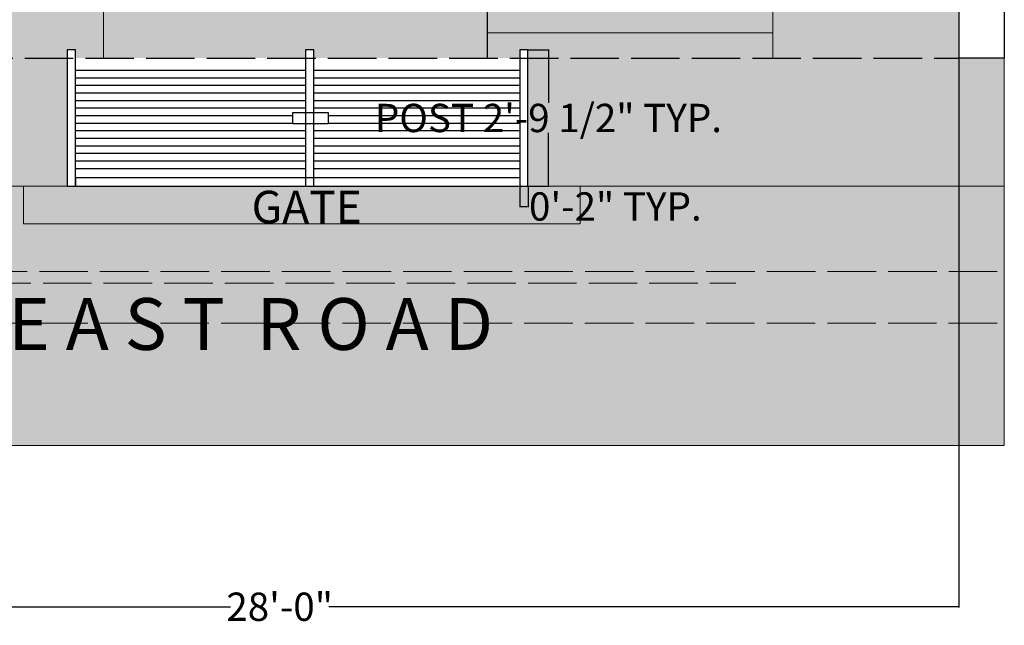
# Model space of a CAD drawing. Units: inches. Extents: x 1316 to 1777, y 813 to 1650.
# Tile 2 of 22: x 1481 to 1724, y 813 to 963. Entities that reach past the tile are written whole.
import ezdxf

# ---------------------------------------------------------------- set-up
doc = ezdxf.new("R2010")
doc.units = ezdxf.units.IN
doc.header["$MEASUREMENT"] = 0
doc.linetypes.add('ACAD_ISO02W100', pattern=[15, 12, -3])
for name, color, linetype, lineweight in [('A-ANNO-DIMS', 2, 'Continuous', 18), ('A-FLOR-STRS', 7, 'Continuous', 25), ('A-FLOR-STRS-PATT', 252, 'Continuous', 13), ('C-PROP', 8, 'ACAD_ISO02W100', 25), ('C-ROAD', 8, 'Continuous', 18), ('C-ROAD-MARK', 9, 'ACAD_ISO02W100', 13), ('C-ROAD-PATT', 251, 'Continuous', 13), ('L-HRDS', 8, 'Continuous', 18), ('L-HRDS-PATT', 252, 'Continuous', 13), ('L-SITE-GATE', 8, 'Continuous', 25), ('text', 7, 'Continuous', 18)]:
    doc.layers.add(name, color=color, linetype=linetype, lineweight=lineweight)
doc.styles.get("Standard").update_dxf_attribs({"font": 'arial.ttf'})
doc.dimstyles.get("Standard").update_dxf_attribs({"dimtxt": 7, "dimasz": 0.18, "dimexe": 0.18, "dimexo": 0.0625, "dimgap": 0.09, "dimtad": 0, "dimtih": 1, "dimtoh": 1, "dimzin": 0, "dimdsep": 46, "dimlunit": 3, "dimtxsty": 'Standard', "dimcen": 0.09, "dimadec": 0, "dimazin": 0, "dimtfac": 1, "dimtofl": 0, "dimtmove": 0, "dimatfit": 3, "dimfxl": 1, "dimtolj": 1, "dimtzin": 0, "dimarcsym": 0})

# ---------------------------------------------------------------- blocks, each defined once
blk = doc.blocks.new('GATE-END-POST')
for p, q in [((2.04, 33.69), (0, 33.69)), ((0, 33.69), (0, 31.67)), ((0, 31.67), (0, 0)), ((2.04, 31.67), (2.04, 33.69)), ((2.04, 0), (2.04, 31.67)), ((0, 0), (2.04, 0))]:
    blk.add_line(p, q)
blk = doc.blocks.new('*D38')
at = {"layer": 'A-ANNO-DIMS', "color": 0, "lineweight": -2, "transparency": 16777216}
for p, q in [((1606.62, 955.71), (1611.79, 955.71)), ((1611.61, 955.53), (1611.61, 942.57)), ((1611.61, 922.2), (1611.61, 935.15)), ((1606.62, 922.02), (1611.79, 922.02))]:
    blk.add_line(p, q, dxfattribs=at)
at = {"layer": 'A-ANNO-DIMS', "color": 0, "transparency": 16777216}
for points in [[(1611.58, 955.53), (1611.64, 955.53), (1611.61, 955.71)], [(1611.58, 922.2), (1611.64, 922.2), (1611.61, 922.02)]]:
    blk.add_solid(points, dxfattribs=at)
at = {"layer": 'Defpoints', "color": 0, "transparency": 16777216}
for p in [(1606.56, 955.71), (1611.61, 955.71), (1606.56, 922.02)]:
    blk.add_point(p, dxfattribs=at)
at = {"layer": 'A-ANNO-DIMS', "color": 0, "transparency": 16777216, "insert": (1611.61, 938.86), "char_height": 7, "attachment_point": 5}
blk.add_mtext('\\A1;POST 2\'-9 1/2" TYP.', dxfattribs=at)
blk = doc.blocks.new('*D39')
at = {"layer": 'A-ANNO-DIMS', "color": 0, "lineweight": -2, "transparency": 16777216}
for p, q in [((1604.52, 921.96), (1604.52, 916.79)), ((1606.56, 921.96), (1606.56, 916.79)), ((1604.7, 916.97), (1606.38, 916.97)), ((1606.56, 916.97), (1606.74, 916.97))]:
    blk.add_line(p, q, dxfattribs=at)
at = {"layer": 'A-ANNO-DIMS', "color": 0, "transparency": 16777216}
for points in [[(1604.7, 917), (1604.7, 916.94), (1604.52, 916.97)], [(1606.38, 917), (1606.38, 916.94), (1606.56, 916.97)]]:
    blk.add_solid(points, dxfattribs=at)
at = {"layer": 'Defpoints', "color": 0, "transparency": 16777216}
for p in [(1604.52, 922.02), (1606.56, 922.02), (1606.56, 916.97)]:
    blk.add_point(p, dxfattribs=at)
at = {"layer": 'A-ANNO-DIMS', "color": 0, "transparency": 16777216, "insert": (1628.17, 916.97), "char_height": 7, "attachment_point": 5}
blk.add_mtext('\\A1;0\'-2" TYP.', dxfattribs=at)
blk = doc.blocks.new('*D50')
at = {"layer": 'A-ANNO-DIMS', "color": 0, "lineweight": -2, "transparency": 16777216}
for p, q in [((1377.06, 1063.81), (1377.06, 817.77)), ((1713.17, 1031.11), (1713.17, 817.77)), ((1377.24, 817.95), (1532.95, 817.95)), ((1712.99, 817.95), (1557.29, 817.95))]:
    blk.add_line(p, q, dxfattribs=at)
at = {"layer": 'A-ANNO-DIMS', "color": 0, "transparency": 16777216}
for points in [[(1377.24, 817.98), (1377.24, 817.92), (1377.06, 817.95)], [(1712.99, 817.98), (1712.99, 817.92), (1713.17, 817.95)]]:
    blk.add_solid(points, dxfattribs=at)
at = {"layer": 'Defpoints', "color": 0, "transparency": 16777216}
for p in [(1377.06, 1063.87), (1713.17, 1031.17), (1713.17, 817.95)]:
    blk.add_point(p, dxfattribs=at)
at = {"layer": 'A-ANNO-DIMS', "color": 0, "transparency": 16777216, "insert": (1545.12, 817.95), "char_height": 7, "attachment_point": 5}
blk.add_mtext('\\A1;28\'-0"', dxfattribs=at)

msp = doc.modelspace()

# ---------------------------------------------------------------- hatches: boundary and pattern name
at = {"layer": 'A-FLOR-STRS-PATT'}
h = msp.add_hatch(color=256, dxfattribs=at)
h.dxf.hatch_style = 1
h.paths.add_polyline_path([(1596.428, 982.68), (1501.564, 982.68), (1501.564, 969.464), (1596.428, 969.464), (1596.428, 971.474)])
h.paths.add_polyline_path([(1596.428, 969.464), (1501.564, 969.464), (1501.564, 965.355), (1501.564, 953.689), (1551.506, 953.689), (1551.506, 955.706), (1553.55, 955.706), (1553.55, 953.689), (1596.428, 953.689)])
at = {"layer": 'C-ROAD-PATT'}
h = msp.add_hatch(color=256, dxfattribs=at)
h.dxf.hatch_style = 1
h.paths.add_polyline_path([(1724.399, 922.018), (1494.583, 922.018), (1365.735, 922.018), (1365.534, 857.849), (1713.173, 857.849), (1724.399, 857.849)])
h = msp.add_hatch(color=256, dxfattribs=at)
h.dxf.hatch_style = 1
h.paths.add_polyline_path([(1724.399, 875.958), (1724.399, 915.982), (1365.716, 915.982), (1365.591, 875.958)])
at = {"layer": 'L-HRDS-PATT'}
h = msp.add_hatch(color=256, dxfattribs=at)
h.dxf.hatch_style = 1
h.paths.add_polyline_path([(1492.539, 953.689), (1377.064, 953.689), (1365.834, 953.689), (1365.735, 922.018), (1492.539, 922.018)])
h.paths.add_polyline_path([(1724.399, 953.689), (1713.173, 953.689), (1606.561, 953.689), (1606.561, 922.018), (1724.399, 922.018)])
h.paths.add_polyline_path([(1667.146, 959.936), (1596.428, 959.936), (1596.428, 953.689), (1604.517, 953.689), (1604.517, 955.706), (1606.561, 955.706), (1606.561, 953.689), (1667.146, 953.689)])
h.paths.add_polyline_path([(1704.173, 1123.869), (1685.903, 1123.869), (1685.903, 1062.613), (1672.026, 1062.613), (1668.679, 1062.613), (1668.679, 1040.173), (1704.173, 1040.173)])
h = msp.add_hatch(color=256, dxfattribs=at)
h.dxf.hatch_style = 1
h.paths.add_polyline_path([(1501.564, 965.355), (1386.064, 965.355), (1386.064, 1063.869), (1377.064, 1063.869), (1377.064, 953.689), (1492.539, 953.689), (1492.539, 955.706), (1494.583, 955.706), (1494.583, 953.689), (1501.564, 953.689)])
h = msp.add_hatch(color=256, dxfattribs=at)
h.dxf.hatch_style = 1
h.paths.add_polyline_path([(1667.146, 1031.173), (1596.428, 1031.173), (1596.428, 982.68), (1596.428, 971.474), (1596.428, 959.936), (1667.146, 959.936)])
h = msp.add_hatch(color=256, dxfattribs=at)
h.dxf.hatch_style = 1
h.paths.add_polyline_path([(1713.173, 1031.173), (1667.146, 1031.173), (1667.146, 953.689), (1713.173, 953.689)])

# ---------------------------------------------------------------- linework, layer by layer
at = {"layer": 'A-FLOR-STRS'}
msp.add_line((1596.428, 971.474), (1596.428, 953.689), dxfattribs=at)
at = {"layer": 'C-PROP'}
for p, q in [((1724.399, 1040.173), (1724.399, 953.689)), ((1377.064, 953.689), (1713.173, 953.689)), ((1724.399, 953.689), (1713.173, 953.689))]:
    msp.add_line(p, q, dxfattribs=at)
at = {"layer": 'C-ROAD'}
for p, q in [((1724.399, 953.689), (1724.399, 857.849)), ((1365.534, 922.018), (1494.583, 922.018)), ((1724.399, 922.018), (1494.583, 922.018)), ((1365.534, 857.849), (1713.173, 857.849)), ((1724.399, 857.849), (1713.173, 857.849))]:
    msp.add_line(p, q, dxfattribs=at)
at = {"layer": 'C-ROAD-MARK'}
for p, q in [((1365.669, 900.851), (1724.399, 900.851)), ((1396.572, 897.973), (1657.977, 897.973)), ((1365.629, 888.109), (1724.399, 888.109))]:
    msp.add_line(p, q, dxfattribs=at)
at = {"layer": 'L-HRDS'}
for p, q in [((1713.173, 953.689), (1713.173, 1040.173)), ((1667.146, 1031.173), (1667.146, 953.689)), ((1501.564, 965.355), (1501.564, 953.689)), ((1596.428, 959.936), (1667.146, 959.936))]:
    msp.add_line(p, q, dxfattribs=at)
at = {"layer": 'L-SITE-GATE'}
for p, q in [((1553.55, 955.706), (1551.506, 955.706)), ((1551.506, 955.706), (1551.506, 953.689)), ((1553.55, 922.018), (1553.55, 955.706)), ((1553.55, 953.689), (1553.55, 955.706)), ((1551.506, 953.689), (1551.506, 922.018)), ((1494.583, 950.698), (1551.506, 950.698)), ((1553.55, 950.698), (1604.517, 950.698)), ((1494.583, 948.828), (1551.506, 948.828)), ((1553.55, 948.828), (1604.517, 948.828)), ((1494.583, 946.958), (1551.506, 946.958)), ((1553.55, 946.958), (1604.517, 946.958)), ((1494.583, 945.088), (1551.506, 945.088)), ((1494.583, 943.218), (1551.506, 943.218)), ((1553.55, 945.088), (1604.517, 945.088)), ((1553.55, 943.218), (1604.517, 943.218)), ((1494.583, 941.347), (1551.506, 941.347)), ((1553.55, 941.347), (1604.517, 941.347)), ((1494.583, 939.477), (1548.36, 939.477)), ((1548.36, 940.207), (1557.156, 940.207)), ((1548.36, 937.411), (1548.36, 940.207)), ((1557.156, 940.207), (1557.156, 937.411)), ((1557.156, 939.477), (1604.517, 939.477)), ((1557.156, 939.477), (1604.517, 939.477)), ((1557.156, 939.477), (1604.517, 939.477)), ((1494.583, 937.607), (1548.36, 937.607)), ((1494.583, 935.737), (1551.506, 935.737)), ((1557.156, 937.411), (1548.36, 937.411)), ((1553.55, 935.737), (1604.517, 935.737)), ((1557.156, 937.607), (1604.517, 937.607)), ((1494.583, 933.866), (1551.506, 933.866)), ((1553.55, 933.866), (1604.517, 933.866)), ((1494.583, 931.996), (1551.506, 931.996)), ((1553.55, 931.996), (1604.517, 931.996)), ((1494.583, 930.126), (1551.506, 930.126)), ((1494.583, 928.256), (1551.506, 928.256)), ((1553.55, 930.126), (1604.517, 930.126)), ((1553.55, 928.256), (1604.517, 928.256)), ((1494.583, 926.385), (1551.506, 926.385)), ((1553.55, 926.385), (1604.517, 926.385)), ((1496.599, 924.062), (1494.583, 924.062)), ((1494.583, 924.062), (1494.583, 922.018)), ((1528.27, 924.062), (1496.599, 924.062)), ((1530.287, 924.062), (1528.27, 924.062)), ((1561.957, 924.062), (1530.287, 924.062)), ((1593.628, 924.062), (1561.957, 924.062)), ((1604.517, 924.062), (1593.628, 924.062)), ((1494.583, 922.018), (1496.599, 922.018)), ((1496.599, 922.018), (1528.27, 922.018)), ((1528.27, 922.018), (1530.287, 922.018)), ((1530.287, 922.018), (1561.957, 922.018)), ((1551.506, 922.018), (1553.55, 922.018)), ((1561.957, 922.018), (1593.628, 922.018)), ((1593.628, 922.018), (1606.561, 922.018))]:
    msp.add_line(p, q, dxfattribs=at)
at = {"layer": 'text'}
for p, q in [((1481.743, 922.018), (1481.743, 912.669)), ((1619.476, 912.669), (1619.476, 922.018)), ((1481.743, 912.669), (1619.476, 912.669))]:
    msp.add_line(p, q, dxfattribs=at)

# ---------------------------------------------------------------- block references
at = {"layer": 'L-SITE-GATE'}
for p in [(1492.539, 922.018), (1604.517, 922.018)]:
    msp.add_blockref('GATE-END-POST', p, dxfattribs=at)

# ---------------------------------------------------------------- texts
at = {"layer": 'text'}
for s, height, p in [('GATE', 8.0489, (1538.179, 912.806)), ('E A S T  R O A D', 12.82247, (1477.977, 881.478))]:
    msp.add_text(s, height=height, dxfattribs=at).set_placement(p)

# ---------------------------------------------------------------- dimensions: what is measured, and where the dimension line sits
at = {"layer": 'A-ANNO-DIMS'}
dim = msp.add_linear_dim(base=(1713.173, 817.949), p1=(1377.064, 1063.869), p2=(1713.173, 1031.173), dimstyle='Standard', override={"dimdec": 1, "dimlfac": 1, "dimrnd": 0, "dimzin": 1, "dimdsep": 46, "dimlunit": 4, "dimfrac": 2}, dxfattribs=at)
dim.commit()
dim.dimension.update_dxf_attribs({"geometry": '*D50', "text_midpoint": (1545.119, 817.949)})
dim = msp.add_linear_dim(base=(1611.614, 955.706), p1=(1606.561, 922.018), p2=(1606.561, 955.706), angle=90, text='POST <> TYP.', dimstyle='Standard', override={"dimdec": 1, "dimlfac": 1, "dimrnd": 0, "dimzin": 1, "dimdsep": 46, "dimlunit": 4, "dimfrac": 2}, dxfattribs=at)
dim.commit()
dim.dimension.update_dxf_attribs({"geometry": '*D38', "text_midpoint": (1611.614, 938.862)})
dim = msp.add_linear_dim(base=(1606.561, 916.965), p1=(1604.517, 922.018), p2=(1606.561, 922.018), text='<> TYP.', dimstyle='Standard', override={"dimdec": 1, "dimlfac": 1, "dimrnd": 0, "dimzin": 1, "dimdsep": 46, "dimlunit": 4, "dimfrac": 2}, dxfattribs=at)
dim.commit()
dim.dimension.update_dxf_attribs({"geometry": '*D39', "text_midpoint": (1628.165, 916.965)})

doc.saveas('drawing.dxf')
